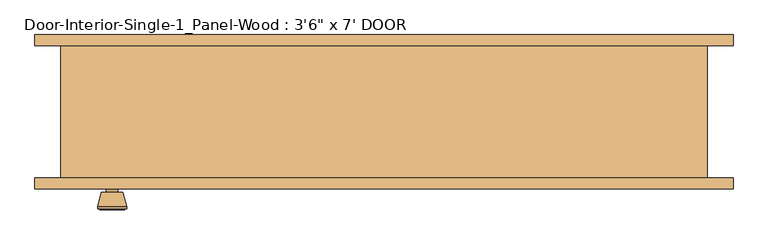
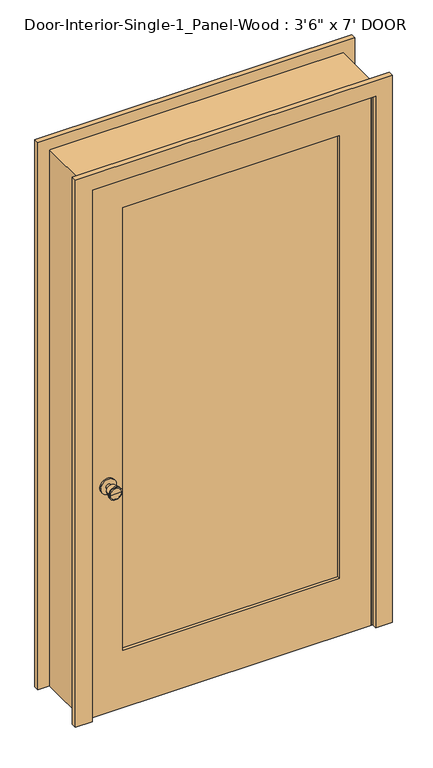
"""IFC4 building model written with IfcOpenShell, lengths in millimetres: door geometry."""

from ifc_helpers import new_model, si_unit, point, frame, frame_2d, origin, place, context, project, spatial, polyline, circle_curve, trimmed, segment, composite_curve, outline, extrude, faceted_brep, source, transform, mapped, element, save
from ifc_brep_helpers import plane_surface, cylinder_surface, revolved_surface, advanced_brep


def door_0f538abb(model_context):
    return source(origin(), model_context, "Body", "SolidModel", [
        advanced_brep(
        [(-469.9, -70.2, 914.4), (-479.9, -70.2, 914.4), (-459.9, -70.2, 914.4), (-449.4241324, -21.2, 914.4), (-490.3758676, -21.2, 914.4), (-469.9, -21.2, 914.4), (-444.9, -23.0278681, 914.4), (-494.9, -23.0278681, 914.4), (-444.9, -26.4915463, 914.4), (-494.9, -26.4915463, 914.4), (-451.263764, -51.2, 914.4), (-488.536236, -51.2, 914.4), (-459.9, -51.2, 914.4), (-479.9, -51.2, 914.4)],
        [
            (0, 1),
            (1, 2, circle_curve(frame((-469.9, -70.2, 914.4), z_axis=(0.0, -1.0, 0.0), x_axis=(-1.0, 0.0, 0.0)), 10.0)),
            (2, 0),
            (2, 1, circle_curve(frame((-469.9, -70.2, 914.4), z_axis=(0.0, -1.0, 0.0), x_axis=(-1.0, 0.0, 0.0)), 10.0)),
            (3, 4, circle_curve(frame((-469.9, -21.2, 914.4), z_axis=(0.0, 1.0, 0.0), x_axis=(-1.0, 0.0, 0.0)), 20.4758676)),
            (4, 5),
            (5, 3),
            (4, 3, circle_curve(frame((-469.9, -21.2, 914.4), z_axis=(0.0, 1.0, 0.0), x_axis=(-1.0, 0.0, 0.0)), 20.4758676)),
            (6, 7, circle_curve(frame((-469.9, -23.0278681, 914.4), z_axis=(0.0, 1.0, 0.0), x_axis=(-1.0, 0.0, 0.0)), 25.0)),
            (7, 4),
            (3, 6),
            (7, 6, circle_curve(frame((-469.9, -23.0278681, 914.4), z_axis=(0.0, 1.0, 0.0), x_axis=(-1.0, 0.0, 0.0)), 25.0)),
            (8, 9, circle_curve(frame((-469.9, -26.4915463, 914.4), z_axis=(0.0, 1.0, 0.0), x_axis=(-1.0, 0.0, 0.0)), 25.0)),
            (9, 7),
            (6, 8),
            (9, 8, circle_curve(frame((-469.9, -26.4915463, 914.4), z_axis=(0.0, 1.0, 0.0), x_axis=(-1.0, 0.0, 0.0)), 25.0)),
            (10, 11, circle_curve(frame((-469.9, -51.2, 914.4), z_axis=(0.0, 1.0, 0.0), x_axis=(-1.0, 0.0, 0.0)), 18.636236)),
            (11, 9),
            (8, 10),
            (11, 10, circle_curve(frame((-469.9, -51.2, 914.4), z_axis=(0.0, 1.0, 0.0), x_axis=(-1.0, 0.0, 0.0)), 18.636236)),
            (12, 13, circle_curve(frame((-469.9, -51.2, 914.4), z_axis=(0.0, 1.0, 0.0), x_axis=(-1.0, 0.0, 0.0)), 10.0)),
            (13, 11),
            (10, 12),
            (13, 12, circle_curve(frame((-469.9, -51.2, 914.4), z_axis=(0.0, 1.0, 0.0), x_axis=(-1.0, 0.0, 0.0)), 10.0)),
            (1, 13),
            (12, 2),
        ],
        [
            plane_surface(frame((-469.9, -70.2, 914.4), z_axis=(0.0, -1.0, 0.0), x_axis=(-1.0, 0.0, 0.0))),
            plane_surface(frame((-469.9, -21.2, 914.4), z_axis=(0.0, 1.0, 0.0), x_axis=(-1.0, 0.0, 0.0))),
            revolved_surface(polyline([(-490.3758676, -21.2, 914.4), (-494.9, -23.0278681, 914.4)]), (-469.9, -70.2, 914.4), (0.0, -1.0, 0.0)),
            cylinder_surface(frame((-469.9, -70.2, 914.4), z_axis=(0.0, -1.0, 0.0), x_axis=(-1.0, 0.0, 0.0)), 25.0),
            revolved_surface(polyline([(-494.9, -26.4915463, 914.4), (-488.536236, -51.2, 914.4)]), (-469.9, -70.2, 914.4), (0.0, -1.0, 0.0)),
            plane_surface(frame((-469.9, -51.2, 914.4), z_axis=(0.0, -1.0, 0.0), x_axis=(-1.0, 0.0, 0.0))),
            cylinder_surface(frame((-469.9, -70.2, 914.4), z_axis=(0.0, -1.0, 0.0), x_axis=(-1.0, 0.0, 0.0)), 10.0),
        ],
        [
            (0, [[1, 2, 3]]),
            (0, [[-3, 4, -1]]),
            (1, [[5, 6, 7]]),
            (1, [[8, -7, -6]]),
            (2, [[9, 10, -5, 11]]),
            (2, [[12, -11, -8, -10]]),
            (3, [[13, 14, -9, 15]]),
            (3, [[16, -15, -12, -14]]),
            (4, [[17, 18, -13, 19]]),
            (4, [[20, -19, -16, -18]]),
            (5, [[21, 22, -17, 23]]),
            (5, [[24, -23, -20, -22]]),
            (6, [[-2, 25, -21, 26]]),
            (6, [[-4, -26, -24, -25]]),
        ],
    ),
        extrude(outline(composite_curve([segment(trimmed(circle_curve(frame_2d((914.4, -469.9)), 30.0), [point((914.4, -499.9))], [point((914.4, -439.9))], False, "CARTESIAN"), True, "CONTINUOUS"), segment(trimmed(circle_curve(frame_2d((914.4, -469.9)), 30.0), [point((914.4, -439.9))], [point((914.4, -499.9))], False, "CARTESIAN"), True, "CONTINUOUS")], self_intersect=False)), frame((0.0, -76.2, 0.0), z_axis=(0.0, 1.0, 0.0), x_axis=(0.0, 0.0, 1.0)), (0.0, 0.0, 1.0), 6.0),
        advanced_brep(
        [(-469.9, -117.125, 914.4), (-459.9, -117.125, 914.4), (-479.9, -117.125, 914.4), (-449.4241324, -166.125, 914.4), (-469.9, -166.125, 914.4), (-490.3758676, -166.125, 914.4), (-444.9, -164.2971319, 914.4), (-494.9, -164.2971319, 914.4), (-444.9, -160.8334537, 914.4), (-494.9, -160.8334537, 914.4), (-451.263764, -136.125, 914.4), (-488.536236, -136.125, 914.4), (-459.9, -136.125, 914.4), (-479.9, -136.125, 914.4)],
        [
            (0, 1),
            (1, 2, circle_curve(frame((-469.9, -117.125, 914.4), z_axis=(0.0, 1.0, 0.0), x_axis=(-1.0, 0.0, 0.0)), 10.0)),
            (2, 0),
            (2, 1, circle_curve(frame((-469.9, -117.125, 914.4), z_axis=(0.0, 1.0, 0.0), x_axis=(-1.0, 0.0, 0.0)), 10.0)),
            (3, 4),
            (4, 5),
            (5, 3, circle_curve(frame((-469.9, -166.125, 914.4), z_axis=(0.0, -1.0, 0.0), x_axis=(-1.0, 0.0, 0.0)), 20.4758676)),
            (3, 5, circle_curve(frame((-469.9, -166.125, 914.4), z_axis=(0.0, -1.0, 0.0), x_axis=(-1.0, 0.0, 0.0)), 20.4758676)),
            (6, 3),
            (5, 7),
            (7, 6, circle_curve(frame((-469.9, -164.2971319, 914.4), z_axis=(0.0, -1.0, 0.0), x_axis=(-1.0, 0.0, 0.0)), 25.0)),
            (6, 7, circle_curve(frame((-469.9, -164.2971319, 914.4), z_axis=(0.0, -1.0, 0.0), x_axis=(-1.0, 0.0, 0.0)), 25.0)),
            (8, 6),
            (7, 9),
            (9, 8, circle_curve(frame((-469.9, -160.8334537, 914.4), z_axis=(0.0, -1.0, 0.0), x_axis=(-1.0, 0.0, 0.0)), 25.0)),
            (8, 9, circle_curve(frame((-469.9, -160.8334537, 914.4), z_axis=(0.0, -1.0, 0.0), x_axis=(-1.0, 0.0, 0.0)), 25.0)),
            (10, 8),
            (9, 11),
            (11, 10, circle_curve(frame((-469.9, -136.125, 914.4), z_axis=(0.0, -1.0, 0.0), x_axis=(-1.0, 0.0, 0.0)), 18.636236)),
            (10, 11, circle_curve(frame((-469.9, -136.125, 914.4), z_axis=(0.0, -1.0, 0.0), x_axis=(-1.0, 0.0, 0.0)), 18.636236)),
            (12, 10),
            (11, 13),
            (13, 12, circle_curve(frame((-469.9, -136.125, 914.4), z_axis=(0.0, -1.0, 0.0), x_axis=(-1.0, 0.0, 0.0)), 10.0)),
            (12, 13, circle_curve(frame((-469.9, -136.125, 914.4), z_axis=(0.0, -1.0, 0.0), x_axis=(-1.0, 0.0, 0.0)), 10.0)),
            (1, 12),
            (13, 2),
        ],
        [
            plane_surface(frame((-469.9, -117.125, 914.4), z_axis=(0.0, 1.0, 0.0), x_axis=(-1.0, 0.0, 0.0))),
            plane_surface(frame((-469.9, -166.125, 914.4), z_axis=(0.0, -1.0, 0.0), x_axis=(-1.0, 0.0, 0.0))),
            revolved_surface(polyline([(-490.3758676, -166.125, 914.4), (-494.9, -164.2971319, 914.4)]), (-469.9, -117.125, 914.4), (0.0, 1.0, 0.0)),
            cylinder_surface(frame((-469.9, -117.125, 914.4), z_axis=(0.0, 1.0, 0.0), x_axis=(-1.0, 0.0, 0.0)), 25.0),
            revolved_surface(polyline([(-494.9, -160.8334537, 914.4), (-488.536236, -136.125, 914.4)]), (-469.9, -117.125, 914.4), (0.0, 1.0, 0.0)),
            plane_surface(frame((-469.9, -136.125, 914.4), z_axis=(0.0, 1.0, 0.0), x_axis=(-1.0, 0.0, 0.0))),
            cylinder_surface(frame((-469.9, -117.125, 914.4), z_axis=(0.0, 1.0, 0.0), x_axis=(-1.0, 0.0, 0.0)), 10.0),
        ],
        [
            (0, [[1, 2, 3]]),
            (0, [[-3, 4, -1]]),
            (1, [[5, 6, 7]]),
            (1, [[-6, -5, 8]]),
            (2, [[9, -7, 10, 11]]),
            (2, [[-10, -8, -9, 12]]),
            (3, [[13, -11, 14, 15]]),
            (3, [[-14, -12, -13, 16]]),
            (4, [[17, -15, 18, 19]]),
            (4, [[-18, -16, -17, 20]]),
            (5, [[21, -19, 22, 23]]),
            (5, [[-22, -20, -21, 24]]),
            (6, [[25, -23, 26, -2]]),
            (6, [[-26, -24, -25, -4]]),
        ],
    ),
        extrude(outline(composite_curve([segment(trimmed(circle_curve(frame_2d((914.4, -469.9)), 30.0), [point((914.4, -499.9))], [point((914.4, -439.9))], False, "CARTESIAN"), True, "CONTINUOUS"), segment(trimmed(circle_curve(frame_2d((914.4, -469.9)), 30.0), [point((914.4, -439.9))], [point((914.4, -499.9))], False, "CARTESIAN"), True, "CONTINUOUS")], self_intersect=False)), frame((0.0, -117.125, 0.0), z_axis=(0.0, 1.0, 0.0), x_axis=(0.0, 0.0, 1.0)), (0.0, 0.0, 1.0), 6.0),
        faceted_brep([(558.8, -111.125, 0.0), (533.4, -111.125, 0.0), (533.4, -76.2, 0.0), (520.7, -76.2, 0.0), (520.7, -41.275, 0.0), (533.4, -41.275, 0.0), (533.4, 117.475, 0.0), (558.8, 117.475, 0.0), (558.8, 117.475, 2159.0), (558.8, -111.125, 2159.0), (533.4, 117.475, 2133.6), (-533.4, 117.475, 2133.6), (-533.4, 117.475, 0.0), (-558.8, 117.475, 0.0), (-558.8, 117.475, 2159.0), (533.4, -41.275, 2133.6), (520.7, -41.275, 2120.9), (-520.7, -41.275, 2120.9), (-520.7, -41.275, 0.0), (-533.4, -41.275, 0.0), (-533.4, -41.275, 2133.6), (520.7, -76.2, 2120.9), (533.4, -76.2, 2133.6), (-533.4, -76.2, 2133.6), (-533.4, -76.2, 0.0), (-520.7, -76.2, 0.0), (-520.7, -76.2, 2120.9), (533.4, -111.125, 2133.6), (-558.8, -111.125, 2159.0), (-558.8, -111.125, 0.0), (-533.4, -111.125, 0.0), (-533.4, -111.125, 2133.6)], [[[0, 1, 2, 3, 4, 5, 6, 7]], [[7, 8, 9, 0]], [[6, 10, 11, 12, 13, 14, 8, 7]], [[5, 15, 10, 6]], [[4, 16, 17, 18, 19, 20, 15, 5]], [[3, 21, 16, 4]], [[2, 22, 23, 24, 25, 26, 21, 3]], [[1, 27, 22, 2]], [[0, 9, 28, 29, 30, 31, 27, 1]], [[8, 14, 28, 9]], [[15, 20, 11, 10]], [[21, 26, 17, 16]], [[27, 31, 23, 22]], [[29, 13, 12, 19, 18, 25, 24, 30]], [[14, 13, 29, 28]], [[20, 19, 12, 11]], [[26, 25, 18, 17]], [[31, 30, 24, 23]]]),
        extrude(outline(polyline([(2133.6, -533.4), (0.0, -533.4), (0.0, 533.4), (2133.6, 533.4), (2133.6, -533.4)]), holes=[polyline([(2014.5375, -412.75), (2014.5375, 412.75), (231.775, 412.75), (231.775, -412.75), (2014.5375, -412.75)])]), frame((0.0, -111.125, 0.0), z_axis=(0.0, 1.0, 0.0), x_axis=(0.0, 0.0, 1.0)), (0.0, 0.0, 1.0), 34.925),
        extrude(outline(polyline([(412.75, -87.8416667), (412.75, -99.4833333), (-412.75, -99.4833333), (-412.75, -87.8416667), (412.75, -87.8416667)])), frame((0.0, 0.0, 231.775), z_axis=(0.0, 0.0, 1.0), x_axis=(1.0, 0.0, 0.0)), (0.0, 0.0, 1.0), 1782.7625),
        extrude(outline(polyline([(0.0, 603.25), (2203.45, 603.25), (2203.45, -603.25), (0.0, -603.25), (0.0, -539.75), (2139.95, -539.75), (2139.95, 539.75), (0.0, 539.75), (0.0, 603.25)])), frame((0.0, -130.175, 0.0), z_axis=(0.0, 1.0, 0.0), x_axis=(0.0, 0.0, 1.0)), (0.0, 0.0, 1.0), 19.05),
        extrude(outline(polyline([(0.0, 603.25), (2203.45, 603.25), (2203.45, -603.25), (0.0, -603.25), (0.0, -539.75), (2139.95, -539.75), (2139.95, 539.75), (0.0, 539.75), (0.0, 603.25)])), frame((0.0, 117.475, 0.0), z_axis=(0.0, 1.0, 0.0), x_axis=(0.0, 0.0, 1.0)), (0.0, 0.0, 1.0), 19.05),
    ])


if __name__ == "__main__":
    model = new_model("IFC4")
    model_context = context("Model", 3, world=origin())
    ifc_project = project(units=[si_unit("LENGTHUNIT", "METRE", prefix="MILLI")], contexts=[model_context])
    site = spatial("IfcSite", under=ifc_project)
    building = spatial("IfcBuilding", under=site)
    placement = place(None, origin())
    door_shape = door_0f538abb(model_context)
    element("IfcDoor", 1, ObjectType="Door-Interior-Single-1_Panel-Wood : 3'6\" x 7' DOOR", at=placement, inside=building, context=model_context, shape_type="MappedRepresentation", body=[
        mapped(door_shape, transform((0.0, 0.0, 0.0), x_axis=(1.0, 0.0, 0.0), y_axis=(0.0, 1.0, 0.0), z_axis=(0.0, 0.0, 1.0))),
    ])
    save(model, "model.ifc")

# Revit data of these elements
# Type "Door-Interior-Single-1_Panel-Wood : 3'6\" x 7' DOOR"
#   Type Mark = "9"
#   Assembly Code = "C1020300"
#   Analytic Construction = "Wooden"
#   Top Rail = 0' - 4 11/16"
#   Thickness = 0' - 1 3/8"
#   Thermal Resistance (R) = 2.5876 (h·ft²·°F)/BTU
#   Swing Angle [instance default] = 90.00°
#   Stiles = 0' - 4 3/4"
#   Rough Width = 3' - 8"
#   Rough Height = 7' - 1"
#   Height = 7' - 0"
#   Width = 3' - 6"
#   Heat Transfer Coefficient (U) = 0.3865 BTU/(h·ft²·°F)
#   Bottom Rail = 0' - 9 1/8"
#   Trim Material = DOOR 3'6" X 7'
#   Panel Material = DOOR 3'6" X 7'
#   Frame Material = DOOR 3'6" X 7'
#   Door Handle Material = Aluminum
#   Visual Light Transmittance = 0
#   Solar Heat Gain Coefficient = 0
#   Wall Closure = (empty or 0)
#   Function = (empty or 0)
# Element 1 (IfcDoor, "Door-Interior-Single-1_Panel-Wood : 3'6\" x 7' DOOR")
#   Materials on its faces: "DOOR 3'6\" X 7'", "Aluminum"
# Materials
#   "DOOR 3'6\" X 7'": class "Generic", colour RGB 120 120 120, transparency 0, Cost = 0
#   "Aluminum": class "Metal", colour RGB 247 247 247, transparency 0, Description = "Aluminum 6061", Cost = 0
